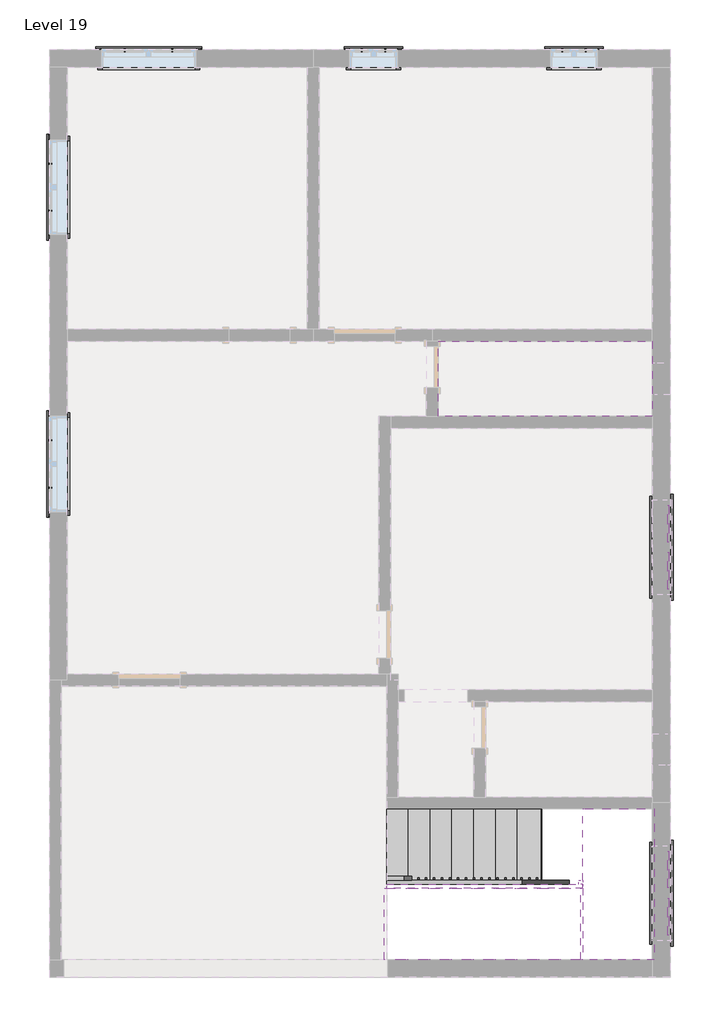
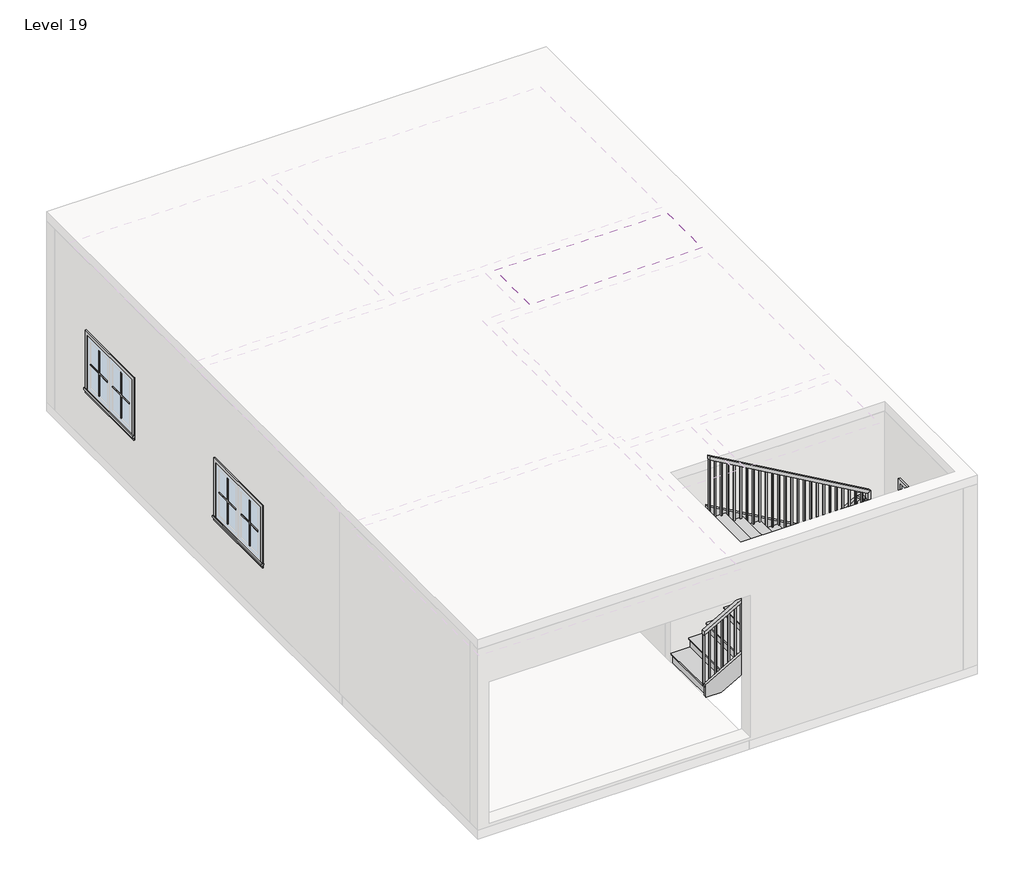
# One storey, part 2 of 2: 44 proxies, 3 members, 2 stair flights, 1 covering, 1 railing, 1 slab.
"""IFC4 building model written with IfcOpenShell, lengths in millimetres."""

from ifc_helpers import new_model, si_unit, frame, origin, place, context, project, spatial, polyline, outline, extrude, faceted_brep, transform, mapped, element, save
from components import muntin_pattern_2x2_muntin_pattern_2x2_2357e71d, muntin_pattern_2x2_muntin_pattern_2x2_302d8f29, muntin_pattern_2x2_muntin_pattern_2x2_53152e2c, muntin_pattern_2x2_muntin_pattern_2x2_e8f3e573, trim_window_exterior_flat_with_sill_c4e67c73, trim_window_exterior_flat_with_sill_a665a915, trim_window_interior_flat_picture_frame_cf1733af, trim_window_interior_flat_picture_frame_d485c387, non_monolithic_landing_13b6ecfc, stair_flight_45c7a08f, stair_flight_466e09e8

model = new_model("IFC4")

# Units and contexts
model_context = context("Model", 3, world=origin())
ifc_project = project(units=[si_unit("LENGTHUNIT", "METRE", prefix="MILLI")], contexts=[model_context])

# Site, building, storey
site = spatial("IfcSite", under=ifc_project)
building = spatial("IfcBuilding", under=site)
storey = spatial("IfcBuildingStorey", under=building, Name="Level 19", Elevation=12801.6)

# Proxies
placement = place(None, origin())
muntin_pattern_2x2_muntin_pattern_2x2_shape = muntin_pattern_2x2_muntin_pattern_2x2_2357e71d(model_context)
element("IfcBuildingElementProxy", 1, Name="Muntin Pattern_2x2 : Muntin Pattern_2x2", ObjectType="Muntin Pattern_2x2 : Muntin Pattern_2x2", at=placement, inside=storey, context=model_context, shape_type="MappedRepresentation", body=[
    mapped(muntin_pattern_2x2_muntin_pattern_2x2_shape, transform((-4942.3279463, 5897.3080275, 13785.85), x_axis=(1.0, 0.0, 0.0), y_axis=(0.0, 1.0, 0.0), z_axis=(0.0, 0.0, 1.0))),
])
element("IfcBuildingElementProxy", 2, Name="Muntin Pattern_2x2 : Muntin Pattern_2x2", ObjectType="Muntin Pattern_2x2 : Muntin Pattern_2x2", at=placement, inside=storey, context=model_context, shape_type="MappedRepresentation", body=[
    mapped(muntin_pattern_2x2_muntin_pattern_2x2_shape, transform((-5899.5904463, 3838.3205275, 13785.85), x_axis=(0.0, 1.0, 0.0), y_axis=(-1.0, 0.0, 0.0), z_axis=(0.0, 0.0, 1.0))),
])
element("IfcBuildingElementProxy", 3, Name="Muntin Pattern_2x2 : Muntin Pattern_2x2", ObjectType="Muntin Pattern_2x2 : Muntin Pattern_2x2", at=placement, inside=storey, context=model_context, shape_type="MappedRepresentation", body=[
    mapped(muntin_pattern_2x2_muntin_pattern_2x2_shape, transform((-5899.5904463, 293.4330275, 13785.85), x_axis=(0.0, 1.0, 0.0), y_axis=(-1.0, 0.0, 0.0), z_axis=(0.0, 0.0, 1.0))),
])
element("IfcBuildingElementProxy", 4, Name="Muntin Pattern_2x2 : Muntin Pattern_2x2", ObjectType="Muntin Pattern_2x2 : Muntin Pattern_2x2", at=placement, inside=storey, context=model_context, shape_type="MappedRepresentation", body=[
    mapped(muntin_pattern_2x2_muntin_pattern_2x2_shape, transform((2031.5595537, -166.9419725, 14090.65), x_axis=(0.0, -1.0, 0.0), y_axis=(1.0, 0.0, 0.0), z_axis=(0.0, 0.0, 1.0))),
])
element("IfcBuildingElementProxy", 5, Name="Muntin Pattern_2x2 : Muntin Pattern_2x2", ObjectType="Muntin Pattern_2x2 : Muntin Pattern_2x2", at=placement, inside=storey, context=model_context, shape_type="MappedRepresentation", body=[
    mapped(muntin_pattern_2x2_muntin_pattern_2x2_shape, transform((2031.5595537, -4599.2419725, 14090.65), x_axis=(0.0, -1.0, 0.0), y_axis=(1.0, 0.0, 0.0), z_axis=(0.0, 0.0, 1.0))),
])
element("IfcBuildingElementProxy", 6, Name="Muntin Pattern_2x2 : Muntin Pattern_2x2", ObjectType="Muntin Pattern_2x2 : Muntin Pattern_2x2", at=placement, inside=storey, context=model_context, shape_type="MappedRepresentation", body=[
    mapped(muntin_pattern_2x2_muntin_pattern_2x2_shape, transform((-4942.3279463, 5897.3080275, 13785.85), x_axis=(1.0, 0.0, 0.0), y_axis=(0.0, 1.0, 0.0), z_axis=(0.0, 0.0, 1.0))),
])
element("IfcBuildingElementProxy", 7, Name="Muntin Pattern_2x2 : Muntin Pattern_2x2", ObjectType="Muntin Pattern_2x2 : Muntin Pattern_2x2", at=placement, inside=storey, context=model_context, shape_type="MappedRepresentation", body=[
    mapped(muntin_pattern_2x2_muntin_pattern_2x2_shape, transform((2031.5595537, -4599.2419725, 14090.65), x_axis=(0.0, -1.0, 0.0), y_axis=(1.0, 0.0, 0.0), z_axis=(0.0, 0.0, 1.0))),
])
muntin_pattern_2x2_muntin_pattern_2x2_2_shape = muntin_pattern_2x2_muntin_pattern_2x2_302d8f29(model_context)
element("IfcBuildingElementProxy", 8, Name="Muntin Pattern_2x2 : Muntin Pattern_2x2", ObjectType="Muntin Pattern_2x2 : Muntin Pattern_2x2", at=placement, inside=storey, context=model_context, shape_type="MappedRepresentation", body=[
    mapped(muntin_pattern_2x2_muntin_pattern_2x2_2_shape, transform((-4335.9029463, 5897.3080275, 13785.85), x_axis=(-1.0, 0.0, 0.0), y_axis=(0.0, -1.0, 0.0), z_axis=(0.0, 0.0, 1.0))),
])
element("IfcBuildingElementProxy", 9, Name="Muntin Pattern_2x2 : Muntin Pattern_2x2", ObjectType="Muntin Pattern_2x2 : Muntin Pattern_2x2", at=placement, inside=storey, context=model_context, shape_type="MappedRepresentation", body=[
    mapped(muntin_pattern_2x2_muntin_pattern_2x2_2_shape, transform((-5899.5904463, 4444.7455275, 13785.85), x_axis=(0.0, -1.0, 0.0), y_axis=(1.0, 0.0, 0.0), z_axis=(0.0, 0.0, 1.0))),
])
element("IfcBuildingElementProxy", 10, Name="Muntin Pattern_2x2 : Muntin Pattern_2x2", ObjectType="Muntin Pattern_2x2 : Muntin Pattern_2x2", at=placement, inside=storey, context=model_context, shape_type="MappedRepresentation", body=[
    mapped(muntin_pattern_2x2_muntin_pattern_2x2_2_shape, transform((-5899.5904463, 899.8580275, 13785.85), x_axis=(0.0, -1.0, 0.0), y_axis=(1.0, 0.0, 0.0), z_axis=(0.0, 0.0, 1.0))),
])
element("IfcBuildingElementProxy", 11, Name="Muntin Pattern_2x2 : Muntin Pattern_2x2", ObjectType="Muntin Pattern_2x2 : Muntin Pattern_2x2", at=placement, inside=storey, context=model_context, shape_type="MappedRepresentation", body=[
    mapped(muntin_pattern_2x2_muntin_pattern_2x2_2_shape, transform((2031.5595537, -773.3669725, 14090.65), x_axis=(0.0, 1.0, 0.0), y_axis=(-1.0, 0.0, 0.0), z_axis=(0.0, 0.0, 1.0))),
])
element("IfcBuildingElementProxy", 12, Name="Muntin Pattern_2x2 : Muntin Pattern_2x2", ObjectType="Muntin Pattern_2x2 : Muntin Pattern_2x2", at=placement, inside=storey, context=model_context, shape_type="MappedRepresentation", body=[
    mapped(muntin_pattern_2x2_muntin_pattern_2x2_2_shape, transform((2031.5595537, -5205.6669725, 14090.65), x_axis=(0.0, 1.0, 0.0), y_axis=(-1.0, 0.0, 0.0), z_axis=(0.0, 0.0, 1.0))),
])
element("IfcBuildingElementProxy", 13, Name="Muntin Pattern_2x2 : Muntin Pattern_2x2", ObjectType="Muntin Pattern_2x2 : Muntin Pattern_2x2", at=placement, inside=storey, context=model_context, shape_type="MappedRepresentation", body=[
    mapped(muntin_pattern_2x2_muntin_pattern_2x2_2_shape, transform((-4335.9029463, 5897.3080275, 13785.85), x_axis=(-1.0, 0.0, 0.0), y_axis=(0.0, -1.0, 0.0), z_axis=(0.0, 0.0, 1.0))),
])
element("IfcBuildingElementProxy", 14, Name="Muntin Pattern_2x2 : Muntin Pattern_2x2", ObjectType="Muntin Pattern_2x2 : Muntin Pattern_2x2", at=placement, inside=storey, context=model_context, shape_type="MappedRepresentation", body=[
    mapped(muntin_pattern_2x2_muntin_pattern_2x2_2_shape, transform((2031.5595537, -5205.6669725, 14090.65), x_axis=(0.0, 1.0, 0.0), y_axis=(-1.0, 0.0, 0.0), z_axis=(0.0, 0.0, 1.0))),
])
muntin_pattern_2x2_muntin_pattern_2x2_3_shape = muntin_pattern_2x2_muntin_pattern_2x2_53152e2c(model_context)
element("IfcBuildingElementProxy", 15, Name="Muntin Pattern_2x2 : Muntin Pattern_2x2", ObjectType="Muntin Pattern_2x2 : Muntin Pattern_2x2", at=placement, inside=storey, context=model_context, shape_type="MappedRepresentation", body=[
    mapped(muntin_pattern_2x2_muntin_pattern_2x2_3_shape, transform((-1907.0279463, 5897.3080275, 13785.85), x_axis=(1.0, 0.0, 0.0), y_axis=(0.0, 1.0, 0.0), z_axis=(0.0, 0.0, 1.0))),
])
element("IfcBuildingElementProxy", 16, Name="Muntin Pattern_2x2 : Muntin Pattern_2x2", ObjectType="Muntin Pattern_2x2 : Muntin Pattern_2x2", at=placement, inside=storey, context=model_context, shape_type="MappedRepresentation", body=[
    mapped(muntin_pattern_2x2_muntin_pattern_2x2_3_shape, transform((658.3720537, 5897.3080275, 13785.85), x_axis=(1.0, 0.0, 0.0), y_axis=(0.0, 1.0, 0.0), z_axis=(0.0, 0.0, 1.0))),
])
element("IfcBuildingElementProxy", 17, Name="Muntin Pattern_2x2 : Muntin Pattern_2x2", ObjectType="Muntin Pattern_2x2 : Muntin Pattern_2x2", at=placement, inside=storey, context=model_context, shape_type="MappedRepresentation", body=[
    mapped(muntin_pattern_2x2_muntin_pattern_2x2_3_shape, transform((-1907.0279463, 5897.3080275, 13785.85), x_axis=(1.0, 0.0, 0.0), y_axis=(0.0, 1.0, 0.0), z_axis=(0.0, 0.0, 1.0))),
])
element("IfcBuildingElementProxy", 18, Name="Muntin Pattern_2x2 : Muntin Pattern_2x2", ObjectType="Muntin Pattern_2x2 : Muntin Pattern_2x2", at=placement, inside=storey, context=model_context, shape_type="MappedRepresentation", body=[
    mapped(muntin_pattern_2x2_muntin_pattern_2x2_3_shape, transform((658.3720537, 5897.3080275, 13785.85), x_axis=(1.0, 0.0, 0.0), y_axis=(0.0, 1.0, 0.0), z_axis=(0.0, 0.0, 1.0))),
])
muntin_pattern_2x2_muntin_pattern_2x2_4_shape = muntin_pattern_2x2_muntin_pattern_2x2_e8f3e573(model_context)
element("IfcBuildingElementProxy", 19, Name="Muntin Pattern_2x2 : Muntin Pattern_2x2", ObjectType="Muntin Pattern_2x2 : Muntin Pattern_2x2", at=placement, inside=storey, context=model_context, shape_type="MappedRepresentation", body=[
    mapped(muntin_pattern_2x2_muntin_pattern_2x2_4_shape, transform((-1605.4029463, 5897.3080275, 13785.85), x_axis=(-1.0, 0.0, 0.0), y_axis=(0.0, -1.0, 0.0), z_axis=(0.0, 0.0, 1.0))),
])
element("IfcBuildingElementProxy", 20, Name="Muntin Pattern_2x2 : Muntin Pattern_2x2", ObjectType="Muntin Pattern_2x2 : Muntin Pattern_2x2", at=placement, inside=storey, context=model_context, shape_type="MappedRepresentation", body=[
    mapped(muntin_pattern_2x2_muntin_pattern_2x2_4_shape, transform((959.9970537, 5897.3080275, 13785.85), x_axis=(-1.0, 0.0, 0.0), y_axis=(0.0, -1.0, 0.0), z_axis=(0.0, 0.0, 1.0))),
])
element("IfcBuildingElementProxy", 21, Name="Muntin Pattern_2x2 : Muntin Pattern_2x2", ObjectType="Muntin Pattern_2x2 : Muntin Pattern_2x2", at=placement, inside=storey, context=model_context, shape_type="MappedRepresentation", body=[
    mapped(muntin_pattern_2x2_muntin_pattern_2x2_4_shape, transform((-1605.4029463, 5897.3080275, 13785.85), x_axis=(-1.0, 0.0, 0.0), y_axis=(0.0, -1.0, 0.0), z_axis=(0.0, 0.0, 1.0))),
])
element("IfcBuildingElementProxy", 22, Name="Muntin Pattern_2x2 : Muntin Pattern_2x2", ObjectType="Muntin Pattern_2x2 : Muntin Pattern_2x2", at=placement, inside=storey, context=model_context, shape_type="MappedRepresentation", body=[
    mapped(muntin_pattern_2x2_muntin_pattern_2x2_4_shape, transform((959.9970537, 5897.3080275, 13785.85), x_axis=(-1.0, 0.0, 0.0), y_axis=(0.0, -1.0, 0.0), z_axis=(0.0, 0.0, 1.0))),
])
trim_window_exterior_flat_with_sill_shape = trim_window_exterior_flat_with_sill_c4e67c73(model_context)
element("IfcBuildingElementProxy", 23, Name="Trim-Window-Exterior-Flat : with Sill", ObjectType="Trim-Window-Exterior-Flat : with Sill", at=placement, inside=storey, context=model_context, shape_type="MappedRepresentation", body=[
    mapped(trim_window_exterior_flat_with_sill_shape, transform((-4639.1154463, 5906.8330275, 14630.4), x_axis=(-1.0, 0.0, 0.0), y_axis=(0.0, 0.0, 1.0), z_axis=(0.0, 1.0, 0.0))),
])
element("IfcBuildingElementProxy", 24, Name="Trim-Window-Exterior-Flat : with Sill", ObjectType="Trim-Window-Exterior-Flat : with Sill", at=placement, inside=storey, context=model_context, shape_type="MappedRepresentation", body=[
    mapped(trim_window_exterior_flat_with_sill_shape, transform((-5909.1154463, 4141.5330275, 14630.4), x_axis=(0.0, -1.0, 0.0), y_axis=(0.0, 0.0, 1.0), z_axis=(-1.0, 0.0, 0.0))),
])
element("IfcBuildingElementProxy", 25, Name="Trim-Window-Exterior-Flat : with Sill", ObjectType="Trim-Window-Exterior-Flat : with Sill", at=placement, inside=storey, context=model_context, shape_type="MappedRepresentation", body=[
    mapped(trim_window_exterior_flat_with_sill_shape, transform((-5909.1154463, 596.6455275, 14630.4), x_axis=(0.0, -1.0, 0.0), y_axis=(0.0, 0.0, 1.0), z_axis=(-1.0, 0.0, 0.0))),
])
element("IfcBuildingElementProxy", 26, Name="Trim-Window-Exterior-Flat : with Sill", ObjectType="Trim-Window-Exterior-Flat : with Sill", at=placement, inside=storey, context=model_context, shape_type="MappedRepresentation", body=[
    mapped(trim_window_exterior_flat_with_sill_shape, transform((2041.0845537, -470.1544725, 14935.2), x_axis=(0.0, 1.0, 0.0), y_axis=(0.0, 0.0, 1.0), z_axis=(1.0, 0.0, 0.0))),
])
element("IfcBuildingElementProxy", 27, Name="Trim-Window-Exterior-Flat : with Sill", ObjectType="Trim-Window-Exterior-Flat : with Sill", at=placement, inside=storey, context=model_context, shape_type="MappedRepresentation", body=[
    mapped(trim_window_exterior_flat_with_sill_shape, transform((2041.0845537, -4902.4544725, 14935.2), x_axis=(0.0, 1.0, 0.0), y_axis=(0.0, 0.0, 1.0), z_axis=(1.0, 0.0, 0.0))),
])
element("IfcBuildingElementProxy", 28, Name="Trim-Window-Exterior-Flat : with Sill", ObjectType="Trim-Window-Exterior-Flat : with Sill", at=placement, inside=storey, context=model_context, shape_type="MappedRepresentation", body=[
    mapped(trim_window_exterior_flat_with_sill_shape, transform((-4639.1154463, 5906.8330275, 14630.4), x_axis=(-1.0, 0.0, 0.0), y_axis=(0.0, 0.0, 1.0), z_axis=(0.0, 1.0, 0.0))),
])
element("IfcBuildingElementProxy", 29, Name="Trim-Window-Exterior-Flat : with Sill", ObjectType="Trim-Window-Exterior-Flat : with Sill", at=placement, inside=storey, context=model_context, shape_type="MappedRepresentation", body=[
    mapped(trim_window_exterior_flat_with_sill_shape, transform((2041.0845537, -4902.4544725, 14935.2), x_axis=(0.0, 1.0, 0.0), y_axis=(0.0, 0.0, 1.0), z_axis=(1.0, 0.0, 0.0))),
])
trim_window_exterior_flat_with_sill_2_shape = trim_window_exterior_flat_with_sill_a665a915(model_context)
element("IfcBuildingElementProxy", 30, Name="Trim-Window-Exterior-Flat : with Sill", ObjectType="Trim-Window-Exterior-Flat : with Sill", at=placement, inside=storey, context=model_context, shape_type="MappedRepresentation", body=[
    mapped(trim_window_exterior_flat_with_sill_2_shape, transform((-1756.2154463, 5906.8330275, 14630.4), x_axis=(-1.0, 0.0, 0.0), y_axis=(0.0, 0.0, 1.0), z_axis=(0.0, 1.0, 0.0))),
])
element("IfcBuildingElementProxy", 31, Name="Trim-Window-Exterior-Flat : with Sill", ObjectType="Trim-Window-Exterior-Flat : with Sill", at=placement, inside=storey, context=model_context, shape_type="MappedRepresentation", body=[
    mapped(trim_window_exterior_flat_with_sill_2_shape, transform((809.1845537, 5906.8330275, 14630.4), x_axis=(-1.0, 0.0, 0.0), y_axis=(0.0, 0.0, 1.0), z_axis=(0.0, 1.0, 0.0))),
])
element("IfcBuildingElementProxy", 32, Name="Trim-Window-Exterior-Flat : with Sill", ObjectType="Trim-Window-Exterior-Flat : with Sill", at=placement, inside=storey, context=model_context, shape_type="MappedRepresentation", body=[
    mapped(trim_window_exterior_flat_with_sill_2_shape, transform((-1756.2154463, 5906.8330275, 14630.4), x_axis=(-1.0, 0.0, 0.0), y_axis=(0.0, 0.0, 1.0), z_axis=(0.0, 1.0, 0.0))),
])
element("IfcBuildingElementProxy", 33, Name="Trim-Window-Exterior-Flat : with Sill", ObjectType="Trim-Window-Exterior-Flat : with Sill", at=placement, inside=storey, context=model_context, shape_type="MappedRepresentation", body=[
    mapped(trim_window_exterior_flat_with_sill_2_shape, transform((809.1845537, 5906.8330275, 14630.4), x_axis=(-1.0, 0.0, 0.0), y_axis=(0.0, 0.0, 1.0), z_axis=(0.0, 1.0, 0.0))),
])
trim_window_interior_flat_picture_frame_shape = trim_window_interior_flat_picture_frame_cf1733af(model_context)
element("IfcBuildingElementProxy", 34, Name="Trim-Window-Interior-Flat : Picture Frame", ObjectType="Trim-Window-Interior-Flat : Picture Frame", at=placement, inside=storey, context=model_context, shape_type="MappedRepresentation", body=[
    mapped(trim_window_interior_flat_picture_frame_shape, transform((-4639.1154463, 5678.2330275, 14630.4), x_axis=(1.0, 0.0, 0.0), y_axis=(0.0, 0.0, 1.0), z_axis=(0.0, -1.0, 0.0))),
])
element("IfcBuildingElementProxy", 35, Name="Trim-Window-Interior-Flat : Picture Frame", ObjectType="Trim-Window-Interior-Flat : Picture Frame", at=placement, inside=storey, context=model_context, shape_type="MappedRepresentation", body=[
    mapped(trim_window_interior_flat_picture_frame_shape, transform((-5680.5154463, 4141.5330275, 14630.4), x_axis=(0.0, 1.0, 0.0), y_axis=(0.0, 0.0, 1.0), z_axis=(1.0, 0.0, 0.0))),
])
element("IfcBuildingElementProxy", 36, Name="Trim-Window-Interior-Flat : Picture Frame", ObjectType="Trim-Window-Interior-Flat : Picture Frame", at=placement, inside=storey, context=model_context, shape_type="MappedRepresentation", body=[
    mapped(trim_window_interior_flat_picture_frame_shape, transform((-5680.5154463, 596.6455275, 14630.4), x_axis=(0.0, 1.0, 0.0), y_axis=(0.0, 0.0, 1.0), z_axis=(1.0, 0.0, 0.0))),
])
element("IfcBuildingElementProxy", 37, Name="Trim-Window-Interior-Flat : Picture Frame", ObjectType="Trim-Window-Interior-Flat : Picture Frame", at=placement, inside=storey, context=model_context, shape_type="MappedRepresentation", body=[
    mapped(trim_window_interior_flat_picture_frame_shape, transform((1812.4845537, -470.1544725, 14935.2), x_axis=(0.0, -1.0, 0.0), y_axis=(0.0, 0.0, 1.0), z_axis=(-1.0, 0.0, 0.0))),
])
element("IfcBuildingElementProxy", 38, Name="Trim-Window-Interior-Flat : Picture Frame", ObjectType="Trim-Window-Interior-Flat : Picture Frame", at=placement, inside=storey, context=model_context, shape_type="MappedRepresentation", body=[
    mapped(trim_window_interior_flat_picture_frame_shape, transform((1812.4845537, -4902.4544725, 14935.2), x_axis=(0.0, -1.0, 0.0), y_axis=(0.0, 0.0, 1.0), z_axis=(-1.0, 0.0, 0.0))),
])
element("IfcBuildingElementProxy", 39, Name="Trim-Window-Interior-Flat : Picture Frame", ObjectType="Trim-Window-Interior-Flat : Picture Frame", at=placement, inside=storey, context=model_context, shape_type="MappedRepresentation", body=[
    mapped(trim_window_interior_flat_picture_frame_shape, transform((-4639.1154463, 5678.2330275, 14630.4), x_axis=(1.0, 0.0, 0.0), y_axis=(0.0, 0.0, 1.0), z_axis=(0.0, -1.0, 0.0))),
])
element("IfcBuildingElementProxy", 40, Name="Trim-Window-Interior-Flat : Picture Frame", ObjectType="Trim-Window-Interior-Flat : Picture Frame", at=placement, inside=storey, context=model_context, shape_type="MappedRepresentation", body=[
    mapped(trim_window_interior_flat_picture_frame_shape, transform((1812.4845537, -4902.4544725, 14935.2), x_axis=(0.0, -1.0, 0.0), y_axis=(0.0, 0.0, 1.0), z_axis=(-1.0, 0.0, 0.0))),
])
trim_window_interior_flat_picture_frame_2_shape = trim_window_interior_flat_picture_frame_d485c387(model_context)
element("IfcBuildingElementProxy", 41, Name="Trim-Window-Interior-Flat : Picture Frame", ObjectType="Trim-Window-Interior-Flat : Picture Frame", at=placement, inside=storey, context=model_context, shape_type="MappedRepresentation", body=[
    mapped(trim_window_interior_flat_picture_frame_2_shape, transform((-1756.2154463, 5678.2330275, 14630.4), x_axis=(1.0, 0.0, 0.0), y_axis=(0.0, 0.0, 1.0), z_axis=(0.0, -1.0, 0.0))),
])
element("IfcBuildingElementProxy", 42, Name="Trim-Window-Interior-Flat : Picture Frame", ObjectType="Trim-Window-Interior-Flat : Picture Frame", at=placement, inside=storey, context=model_context, shape_type="MappedRepresentation", body=[
    mapped(trim_window_interior_flat_picture_frame_2_shape, transform((809.1845537, 5678.2330275, 14630.4), x_axis=(1.0, 0.0, 0.0), y_axis=(0.0, 0.0, 1.0), z_axis=(0.0, -1.0, 0.0))),
])
element("IfcBuildingElementProxy", 43, Name="Trim-Window-Interior-Flat : Picture Frame", ObjectType="Trim-Window-Interior-Flat : Picture Frame", at=placement, inside=storey, context=model_context, shape_type="MappedRepresentation", body=[
    mapped(trim_window_interior_flat_picture_frame_2_shape, transform((-1756.2154463, 5678.2330275, 14630.4), x_axis=(1.0, 0.0, 0.0), y_axis=(0.0, 0.0, 1.0), z_axis=(0.0, -1.0, 0.0))),
])
element("IfcBuildingElementProxy", 44, Name="Trim-Window-Interior-Flat : Picture Frame", ObjectType="Trim-Window-Interior-Flat : Picture Frame", at=placement, inside=storey, context=model_context, shape_type="MappedRepresentation", body=[
    mapped(trim_window_interior_flat_picture_frame_2_shape, transform((809.1845537, 5678.2330275, 14630.4), x_axis=(1.0, 0.0, 0.0), y_axis=(0.0, 0.0, 1.0), z_axis=(0.0, -1.0, 0.0))),
])

# Covering
element("IfcCovering", 45, ObjectType="2' x 4' ACT System", at=placement, inside=storey, context=model_context, shape_type="SweptSolid", body=[
    extrude(outline(polyline([(-930.7154463, 2171.4455275), (1812.4845537, 2171.4455275), (1812.4845537, 1206.2455275), (-930.7154463, 1206.2455275), (-930.7154463, 2171.4455275)])), frame((0.0, 0.0, 15544.8), z_axis=(0.0, 0.0, 1.0), x_axis=(1.0, 0.0, 0.0)), (0.0, 0.0, 1.0), 57.15),
])

# Members
element("IfcMember", 46, ObjectType="Stringer - 2\" Width", at=placement, inside=storey, context=model_context, shape_type="SweptSolid", body=[
    extrude(outline(polyline([(13010.6890626, -1591.1154463), (12801.6, -1591.1154463), (12801.6, -1342.8974141), (14070.524218, 872.6845537), (14421.7745172, 872.6845537), (13010.6890626, -1591.1154463)])), frame((0.0, -4788.1544725, 0.0), z_axis=(0.0, 1.0, 0.0), x_axis=(0.0, 0.0, 1.0)), (0.0, 0.0, 1.0), 50.8),
])
element("IfcMember", 47, ObjectType="Stringer - 2\" Width", at=placement, inside=storey, context=model_context, shape_type="SweptSolid", body=[
    extrude(outline(polyline([(14259.6387634, 923.4845537), (14610.8890626, 923.4845537), (16051.0690626, -1591.1154463), (15699.8187634, -1591.1154463), (14259.6387634, 923.4845537)])), frame((0.0, -4838.9544725, 0.0), z_axis=(0.0, 1.0, 0.0), x_axis=(0.0, 0.0, 1.0)), (0.0, 0.0, 1.0), 50.8),
])
element("IfcMember", 48, ObjectType="Stringer - 2\" Width", at=placement, inside=storey, context=model_context, shape_type="SweptSolid", body=[
    extrude(outline(polyline([(872.6845537, -4737.3544725), (923.4845537, -4737.3544725), (923.4845537, -4788.1544725), (872.6845537, -4788.1544725), (872.6845537, -4737.3544725)])), frame((0.0, 0.0, 14173.2), z_axis=(0.0, 0.0, 1.0), x_axis=(1.0, 0.0, 0.0)), (0.0, 0.0, 1.0), 304.8),
])

# Railing
element("IfcRailing", 49, ObjectType="Handrail - Rectangular", at=placement, inside=storey, context=model_context, shape_type="SolidModel", body=[
    faceted_brep([(-1591.1154463, -4686.5544725, 13876.02), (-1591.1154463, -4686.5544725, 13817.4782835), (-1591.1154463, -4737.3544725, 13817.4782835), (-1591.1154463, -4737.3544725, 13876.02), (847.2845537, -4686.5544725, 15272.5581818), (898.0845537, -4686.5544725, 15243.1110107), (898.0845537, -4737.3544725, 15243.1110107), (847.2845537, -4737.3544725, 15272.5581818), (847.2845537, -4686.5544725, 15316.2), (898.0845537, -4686.5544725, 15265.4), (898.0845537, -4737.3544725, 15265.4), (847.2845537, -4737.3544725, 15316.2), (974.2845537, -4686.5544725, 15316.2), (974.2845537, -4686.5544725, 15265.4), (923.4845537, -4737.3544725, 15265.4), (923.4845537, -4737.3544725, 15316.2), (974.2845537, -4813.5544725, 15316.2), (974.2845537, -4813.5544725, 15265.4), (923.4845537, -4813.5544725, 15265.4), (923.4845537, -4813.5544725, 15316.2), (974.2845537, -4838.9544725, 15316.2), (923.4845537, -4838.9544725, 15316.2), (923.4845537, -4889.7544725, 15265.4), (974.2845537, -4889.7544725, 15265.4)], [[[0, 1, 2, 3]], [[1, 0, 4, 5]], [[2, 1, 5, 6]], [[3, 2, 6, 7]], [[0, 3, 7, 4]], [[5, 4, 8, 9]], [[6, 5, 9, 10]], [[7, 6, 10, 11]], [[4, 7, 11, 8]], [[9, 8, 12, 13]], [[10, 9, 13, 14]], [[11, 10, 14, 15]], [[8, 11, 15, 12]], [[13, 12, 16, 17]], [[14, 13, 17, 18]], [[15, 14, 18, 19]], [[12, 15, 19, 16]], [[20, 21, 22, 23]], [[17, 16, 20, 23]], [[18, 17, 23, 22]], [[19, 18, 22, 21]], [[16, 19, 21, 20]]]),
    faceted_brep([(974.2845537, -4838.9544725, 15316.2), (974.2845537, -4889.7544725, 15265.4), (923.4845537, -4889.7544725, 15265.4), (923.4845537, -4838.9544725, 15316.2), (974.2845537, -4838.9544725, 15447.1254545), (923.4845537, -4838.9544725, 15417.6782835), (923.4845537, -4889.7544725, 15417.6782835), (974.2845537, -4889.7544725, 15447.1254545)], [[[0, 1, 2, 3]], [[4, 5, 6, 7]], [[1, 0, 4, 7]], [[2, 1, 7, 6]], [[3, 2, 6, 5]], [[0, 3, 5, 4]]]),
    faceted_brep([(974.2845537, -4889.7544725, 15447.1254545), (923.4845537, -4889.7544725, 15417.6782835), (923.4845537, -4838.9544725, 15417.6782835), (974.2845537, -4838.9544725, 15447.1254545), (-1591.1154463, -4889.7544725, 16916.4), (-1591.1154463, -4838.9544725, 16916.4), (-1591.1154463, -4838.9544725, 16857.8582835), (-1591.1154463, -4889.7544725, 16857.8582835)], [[[0, 1, 2, 3]], [[4, 5, 6, 7]], [[1, 0, 4, 7]], [[2, 1, 7, 6]], [[3, 2, 6, 5]], [[0, 3, 5, 4]]]),
    extrude(outline(polyline([(16794.2139653, -1479.9904463), (16805.1244198, -1499.0404463), (15841.98, -1499.0404463), (15841.98, -1479.9904463), (16794.2139653, -1479.9904463)])), frame((0.0, -4873.8794725, 0.0), z_axis=(0.0, 1.0, 0.0), x_axis=(0.0, 0.0, 1.0)), (0.0, 0.0, 1.0), 19.05),
    extrude(outline(polyline([(16736.0248744, -1378.3904463), (16746.9353289, -1397.4404463), (15841.98, -1397.4404463), (15841.98, -1378.3904463), (16736.0248744, -1378.3904463)])), frame((0.0, -4873.8794725, 0.0), z_axis=(0.0, 1.0, 0.0), x_axis=(0.0, 0.0, 1.0)), (0.0, 0.0, 1.0), 19.05),
    extrude(outline(polyline([(16677.8357835, -1276.7904463), (16688.746238, -1295.8404463), (15681.96, -1295.8404463), (15681.96, -1276.7904463), (16677.8357835, -1276.7904463)])), frame((0.0, -4873.8794725, 0.0), z_axis=(0.0, 1.0, 0.0), x_axis=(0.0, 0.0, 1.0)), (0.0, 0.0, 1.0), 19.05),
    extrude(outline(polyline([(16619.6466926, -1175.1904463), (16630.5571471, -1194.2404463), (15681.96, -1194.2404463), (15681.96, -1175.1904463), (16619.6466926, -1175.1904463)])), frame((0.0, -4873.8794725, 0.0), z_axis=(0.0, 1.0, 0.0), x_axis=(0.0, 0.0, 1.0)), (0.0, 0.0, 1.0), 19.05),
    extrude(outline(polyline([(16561.4576016, -1073.5904463), (16572.3680562, -1092.6404463), (15681.96, -1092.6404463), (15681.96, -1073.5904463), (16561.4576016, -1073.5904463)])), frame((0.0, -4873.8794725, 0.0), z_axis=(0.0, 1.0, 0.0), x_axis=(0.0, 0.0, 1.0)), (0.0, 0.0, 1.0), 19.05),
    extrude(outline(polyline([(16503.2685107, -971.9904463), (16514.1789653, -991.0404463), (15521.94, -991.0404463), (15521.94, -971.9904463), (16503.2685107, -971.9904463)])), frame((0.0, -4873.8794725, 0.0), z_axis=(0.0, 1.0, 0.0), x_axis=(0.0, 0.0, 1.0)), (0.0, 0.0, 1.0), 19.05),
    extrude(outline(polyline([(16445.0794198, -870.3904463), (16455.9898744, -889.4404463), (15521.94, -889.4404463), (15521.94, -870.3904463), (16445.0794198, -870.3904463)])), frame((0.0, -4873.8794725, 0.0), z_axis=(0.0, 1.0, 0.0), x_axis=(0.0, 0.0, 1.0)), (0.0, 0.0, 1.0), 19.05),
    extrude(outline(polyline([(16386.8903289, -768.7904463), (16397.8007835, -787.8404463), (15521.94, -787.8404463), (15521.94, -768.7904463), (16386.8903289, -768.7904463)])), frame((0.0, -4873.8794725, 0.0), z_axis=(0.0, 1.0, 0.0), x_axis=(0.0, 0.0, 1.0)), (0.0, 0.0, 1.0), 19.05),
    extrude(outline(polyline([(16328.701238, -667.1904463), (16339.6116926, -686.2404463), (15361.92, -686.2404463), (15361.92, -667.1904463), (16328.701238, -667.1904463)])), frame((0.0, -4873.8794725, 0.0), z_axis=(0.0, 1.0, 0.0), x_axis=(0.0, 0.0, 1.0)), (0.0, 0.0, 1.0), 19.05),
    extrude(outline(polyline([(16270.5121471, -565.5904463), (16281.4226016, -584.6404463), (15361.92, -584.6404463), (15361.92, -565.5904463), (16270.5121471, -565.5904463)])), frame((0.0, -4873.8794725, 0.0), z_axis=(0.0, 1.0, 0.0), x_axis=(0.0, 0.0, 1.0)), (0.0, 0.0, 1.0), 19.05),
    extrude(outline(polyline([(16212.3230562, -463.9904463), (16223.2335107, -483.0404463), (15361.92, -483.0404463), (15361.92, -463.9904463), (16212.3230562, -463.9904463)])), frame((0.0, -4873.8794725, 0.0), z_axis=(0.0, 1.0, 0.0), x_axis=(0.0, 0.0, 1.0)), (0.0, 0.0, 1.0), 19.05),
    extrude(outline(polyline([(16154.1339653, -362.3904463), (16165.0444198, -381.4404463), (15201.9, -381.4404463), (15201.9, -362.3904463), (16154.1339653, -362.3904463)])), frame((0.0, -4873.8794725, 0.0), z_axis=(0.0, 1.0, 0.0), x_axis=(0.0, 0.0, 1.0)), (0.0, 0.0, 1.0), 19.05),
    extrude(outline(polyline([(16095.9448744, -260.7904463), (16106.8553289, -279.8404463), (15201.9, -279.8404463), (15201.9, -260.7904463), (16095.9448744, -260.7904463)])), frame((0.0, -4873.8794725, 0.0), z_axis=(0.0, 1.0, 0.0), x_axis=(0.0, 0.0, 1.0)), (0.0, 0.0, 1.0), 19.05),
    extrude(outline(polyline([(16037.7557835, -159.1904463), (16048.666238, -178.2404463), (15041.88, -178.2404463), (15041.88, -159.1904463), (16037.7557835, -159.1904463)])), frame((0.0, -4873.8794725, 0.0), z_axis=(0.0, 1.0, 0.0), x_axis=(0.0, 0.0, 1.0)), (0.0, 0.0, 1.0), 19.05),
    extrude(outline(polyline([(15979.5666926, -57.5904463), (15990.4771471, -76.6404463), (15041.88, -76.6404463), (15041.88, -57.5904463), (15979.5666926, -57.5904463)])), frame((0.0, -4873.8794725, 0.0), z_axis=(0.0, 1.0, 0.0), x_axis=(0.0, 0.0, 1.0)), (0.0, 0.0, 1.0), 19.05),
    extrude(outline(polyline([(15921.3776016, 44.0095537), (15932.2880562, 24.9595537), (15041.88, 24.9595537), (15041.88, 44.0095537), (15921.3776016, 44.0095537)])), frame((0.0, -4873.8794725, 0.0), z_axis=(0.0, 1.0, 0.0), x_axis=(0.0, 0.0, 1.0)), (0.0, 0.0, 1.0), 19.05),
    extrude(outline(polyline([(15863.1885107, 145.6095537), (15874.0989653, 126.5595537), (14881.86, 126.5595537), (14881.86, 145.6095537), (15863.1885107, 145.6095537)])), frame((0.0, -4873.8794725, 0.0), z_axis=(0.0, 1.0, 0.0), x_axis=(0.0, 0.0, 1.0)), (0.0, 0.0, 1.0), 19.05),
    extrude(outline(polyline([(15804.9994198, 247.2095537), (15815.9098744, 228.1595537), (14881.86, 228.1595537), (14881.86, 247.2095537), (15804.9994198, 247.2095537)])), frame((0.0, -4873.8794725, 0.0), z_axis=(0.0, 1.0, 0.0), x_axis=(0.0, 0.0, 1.0)), (0.0, 0.0, 1.0), 19.05),
    extrude(outline(polyline([(15746.8103289, 348.8095537), (15757.7207835, 329.7595537), (14881.86, 329.7595537), (14881.86, 348.8095537), (15746.8103289, 348.8095537)])), frame((0.0, -4873.8794725, 0.0), z_axis=(0.0, 1.0, 0.0), x_axis=(0.0, 0.0, 1.0)), (0.0, 0.0, 1.0), 19.05),
    extrude(outline(polyline([(15688.621238, 450.4095537), (15699.5316926, 431.3595537), (14721.84, 431.3595537), (14721.84, 450.4095537), (15688.621238, 450.4095537)])), frame((0.0, -4873.8794725, 0.0), z_axis=(0.0, 1.0, 0.0), x_axis=(0.0, 0.0, 1.0)), (0.0, 0.0, 1.0), 19.05),
    extrude(outline(polyline([(15630.4321471, 552.0095537), (15641.3426016, 532.9595537), (14721.84, 532.9595537), (14721.84, 552.0095537), (15630.4321471, 552.0095537)])), frame((0.0, -4873.8794725, 0.0), z_axis=(0.0, 1.0, 0.0), x_axis=(0.0, 0.0, 1.0)), (0.0, 0.0, 1.0), 19.05),
    extrude(outline(polyline([(15572.2430562, 653.6095537), (15583.1535107, 634.5595537), (14721.84, 634.5595537), (14721.84, 653.6095537), (15572.2430562, 653.6095537)])), frame((0.0, -4873.8794725, 0.0), z_axis=(0.0, 1.0, 0.0), x_axis=(0.0, 0.0, 1.0)), (0.0, 0.0, 1.0), 19.05),
    extrude(outline(polyline([(15514.0539653, 755.2095537), (15524.9644198, 736.1595537), (14561.82, 736.1595537), (14561.82, 755.2095537), (15514.0539653, 755.2095537)])), frame((0.0, -4873.8794725, 0.0), z_axis=(0.0, 1.0, 0.0), x_axis=(0.0, 0.0, 1.0)), (0.0, 0.0, 1.0), 19.05),
    extrude(outline(polyline([(15455.8648744, 856.8095537), (15466.7753289, 837.7595537), (14561.82, 837.7595537), (14561.82, 856.8095537), (15455.8648744, 856.8095537)])), frame((0.0, -4873.8794725, 0.0), z_axis=(0.0, 1.0, 0.0), x_axis=(0.0, 0.0, 1.0)), (0.0, 0.0, 1.0), 19.05),
    extrude(outline(polyline([(939.3595537, -4804.0294725), (958.4095537, -4804.0294725), (958.4095537, -4823.0794725), (939.3595537, -4823.0794725), (939.3595537, -4804.0294725)])), frame((0.0, 0.0, 14401.8), z_axis=(0.0, 0.0, 1.0), x_axis=(1.0, 0.0, 0.0)), (0.0, 0.0, 1.0), 863.6),
    extrude(outline(polyline([(15219.4716926, 856.8095537), (15208.561238, 837.7595537), (14241.78, 837.7595537), (14241.78, 856.8095537), (15219.4716926, 856.8095537)])), frame((0.0, -4721.4794725, 0.0), z_axis=(0.0, 1.0, 0.0), x_axis=(0.0, 0.0, 1.0)), (0.0, 0.0, 1.0), 19.05),
    extrude(outline(polyline([(15161.2826016, 755.2095537), (15150.3721471, 736.1595537), (14241.78, 736.1595537), (14241.78, 755.2095537), (15161.2826016, 755.2095537)])), frame((0.0, -4721.4794725, 0.0), z_axis=(0.0, 1.0, 0.0), x_axis=(0.0, 0.0, 1.0)), (0.0, 0.0, 1.0), 19.05),
    extrude(outline(polyline([(15103.0935107, 653.6095537), (15092.1830562, 634.5595537), (14241.78, 634.5595537), (14241.78, 653.6095537), (15103.0935107, 653.6095537)])), frame((0.0, -4721.4794725, 0.0), z_axis=(0.0, 1.0, 0.0), x_axis=(0.0, 0.0, 1.0)), (0.0, 0.0, 1.0), 19.05),
    extrude(outline(polyline([(15044.9044198, 552.0095537), (15033.9939653, 532.9595537), (14081.76, 532.9595537), (14081.76, 552.0095537), (15044.9044198, 552.0095537)])), frame((0.0, -4721.4794725, 0.0), z_axis=(0.0, 1.0, 0.0), x_axis=(0.0, 0.0, 1.0)), (0.0, 0.0, 1.0), 19.05),
    extrude(outline(polyline([(14986.7153289, 450.4095537), (14975.8048744, 431.3595537), (14081.76, 431.3595537), (14081.76, 450.4095537), (14986.7153289, 450.4095537)])), frame((0.0, -4721.4794725, 0.0), z_axis=(0.0, 1.0, 0.0), x_axis=(0.0, 0.0, 1.0)), (0.0, 0.0, 1.0), 19.05),
    extrude(outline(polyline([(14928.526238, 348.8095537), (14917.6157835, 329.7595537), (13921.74, 329.7595537), (13921.74, 348.8095537), (14928.526238, 348.8095537)])), frame((0.0, -4721.4794725, 0.0), z_axis=(0.0, 1.0, 0.0), x_axis=(0.0, 0.0, 1.0)), (0.0, 0.0, 1.0), 19.05),
    extrude(outline(polyline([(14870.3371471, 247.2095537), (14859.4266926, 228.1595537), (13921.74, 228.1595537), (13921.74, 247.2095537), (14870.3371471, 247.2095537)])), frame((0.0, -4721.4794725, 0.0), z_axis=(0.0, 1.0, 0.0), x_axis=(0.0, 0.0, 1.0)), (0.0, 0.0, 1.0), 19.05),
    extrude(outline(polyline([(14812.1480562, 145.6095537), (14801.2376016, 126.5595537), (13921.74, 126.5595537), (13921.74, 145.6095537), (14812.1480562, 145.6095537)])), frame((0.0, -4721.4794725, 0.0), z_axis=(0.0, 1.0, 0.0), x_axis=(0.0, 0.0, 1.0)), (0.0, 0.0, 1.0), 19.05),
    extrude(outline(polyline([(14753.9589653, 44.0095537), (14743.0485107, 24.9595537), (13761.72, 24.9595537), (13761.72, 44.0095537), (14753.9589653, 44.0095537)])), frame((0.0, -4721.4794725, 0.0), z_axis=(0.0, 1.0, 0.0), x_axis=(0.0, 0.0, 1.0)), (0.0, 0.0, 1.0), 19.05),
    extrude(outline(polyline([(14695.7698744, -57.5904463), (14684.8594198, -76.6404463), (13761.72, -76.6404463), (13761.72, -57.5904463), (14695.7698744, -57.5904463)])), frame((0.0, -4721.4794725, 0.0), z_axis=(0.0, 1.0, 0.0), x_axis=(0.0, 0.0, 1.0)), (0.0, 0.0, 1.0), 19.05),
    extrude(outline(polyline([(14637.5807835, -159.1904463), (14626.6703289, -178.2404463), (13761.72, -178.2404463), (13761.72, -159.1904463), (14637.5807835, -159.1904463)])), frame((0.0, -4721.4794725, 0.0), z_axis=(0.0, 1.0, 0.0), x_axis=(0.0, 0.0, 1.0)), (0.0, 0.0, 1.0), 19.05),
    extrude(outline(polyline([(14579.3916926, -260.7904463), (14568.481238, -279.8404463), (13601.7, -279.8404463), (13601.7, -260.7904463), (14579.3916926, -260.7904463)])), frame((0.0, -4721.4794725, 0.0), z_axis=(0.0, 1.0, 0.0), x_axis=(0.0, 0.0, 1.0)), (0.0, 0.0, 1.0), 19.05),
    extrude(outline(polyline([(14521.2026016, -362.3904463), (14510.2921471, -381.4404463), (13601.7, -381.4404463), (13601.7, -362.3904463), (14521.2026016, -362.3904463)])), frame((0.0, -4721.4794725, 0.0), z_axis=(0.0, 1.0, 0.0), x_axis=(0.0, 0.0, 1.0)), (0.0, 0.0, 1.0), 19.05),
    extrude(outline(polyline([(14463.0135107, -463.9904463), (14452.1030562, -483.0404463), (13601.7, -483.0404463), (13601.7, -463.9904463), (14463.0135107, -463.9904463)])), frame((0.0, -4721.4794725, 0.0), z_axis=(0.0, 1.0, 0.0), x_axis=(0.0, 0.0, 1.0)), (0.0, 0.0, 1.0), 19.05),
    extrude(outline(polyline([(14404.8244198, -565.5904463), (14393.9139653, -584.6404463), (13441.68, -584.6404463), (13441.68, -565.5904463), (14404.8244198, -565.5904463)])), frame((0.0, -4721.4794725, 0.0), z_axis=(0.0, 1.0, 0.0), x_axis=(0.0, 0.0, 1.0)), (0.0, 0.0, 1.0), 19.05),
    extrude(outline(polyline([(14346.6353289, -667.1904463), (14335.7248744, -686.2404463), (13441.68, -686.2404463), (13441.68, -667.1904463), (14346.6353289, -667.1904463)])), frame((0.0, -4721.4794725, 0.0), z_axis=(0.0, 1.0, 0.0), x_axis=(0.0, 0.0, 1.0)), (0.0, 0.0, 1.0), 19.05),
    extrude(outline(polyline([(14288.446238, -768.7904463), (14277.5357835, -787.8404463), (13281.66, -787.8404463), (13281.66, -768.7904463), (14288.446238, -768.7904463)])), frame((0.0, -4721.4794725, 0.0), z_axis=(0.0, 1.0, 0.0), x_axis=(0.0, 0.0, 1.0)), (0.0, 0.0, 1.0), 19.05),
    extrude(outline(polyline([(14230.2571471, -870.3904463), (14219.3466926, -889.4404463), (13281.66, -889.4404463), (13281.66, -870.3904463), (14230.2571471, -870.3904463)])), frame((0.0, -4721.4794725, 0.0), z_axis=(0.0, 1.0, 0.0), x_axis=(0.0, 0.0, 1.0)), (0.0, 0.0, 1.0), 19.05),
    extrude(outline(polyline([(14172.0680562, -971.9904463), (14161.1576016, -991.0404463), (13281.66, -991.0404463), (13281.66, -971.9904463), (14172.0680562, -971.9904463)])), frame((0.0, -4721.4794725, 0.0), z_axis=(0.0, 1.0, 0.0), x_axis=(0.0, 0.0, 1.0)), (0.0, 0.0, 1.0), 19.05),
    extrude(outline(polyline([(14113.8789653, -1073.5904463), (14102.9685107, -1092.6404463), (13121.64, -1092.6404463), (13121.64, -1073.5904463), (14113.8789653, -1073.5904463)])), frame((0.0, -4721.4794725, 0.0), z_axis=(0.0, 1.0, 0.0), x_axis=(0.0, 0.0, 1.0)), (0.0, 0.0, 1.0), 19.05),
    extrude(outline(polyline([(14055.6898744, -1175.1904463), (14044.7794198, -1194.2404463), (13121.64, -1194.2404463), (13121.64, -1175.1904463), (14055.6898744, -1175.1904463)])), frame((0.0, -4721.4794725, 0.0), z_axis=(0.0, 1.0, 0.0), x_axis=(0.0, 0.0, 1.0)), (0.0, 0.0, 1.0), 19.05),
    extrude(outline(polyline([(13997.5007835, -1276.7904463), (13986.5903289, -1295.8404463), (13121.64, -1295.8404463), (13121.64, -1276.7904463), (13997.5007835, -1276.7904463)])), frame((0.0, -4721.4794725, 0.0), z_axis=(0.0, 1.0, 0.0), x_axis=(0.0, 0.0, 1.0)), (0.0, 0.0, 1.0), 19.05),
    extrude(outline(polyline([(13939.3116926, -1378.3904463), (13928.401238, -1397.4404463), (12961.62, -1397.4404463), (12961.62, -1378.3904463), (13939.3116926, -1378.3904463)])), frame((0.0, -4721.4794725, 0.0), z_axis=(0.0, 1.0, 0.0), x_axis=(0.0, 0.0, 1.0)), (0.0, 0.0, 1.0), 19.05),
    extrude(outline(polyline([(13881.1226016, -1479.9904463), (13870.2121471, -1499.0404463), (12961.62, -1499.0404463), (12961.62, -1479.9904463), (13881.1226016, -1479.9904463)])), frame((0.0, -4721.4794725, 0.0), z_axis=(0.0, 1.0, 0.0), x_axis=(0.0, 0.0, 1.0)), (0.0, 0.0, 1.0), 19.05),
    extrude(outline(polyline([(939.3595537, -4854.8294725), (958.4095537, -4854.8294725), (958.4095537, -4873.8794725), (939.3595537, -4873.8794725), (939.3595537, -4854.8294725)])), frame((0.0, 0.0, 14401.8), z_axis=(0.0, 0.0, 1.0), x_axis=(1.0, 0.0, 0.0)), (0.0, 0.0, 1.0), 863.6),
    extrude(outline(polyline([(939.3595537, -4721.4794725), (939.3595537, -4702.4294725), (958.4095537, -4702.4294725), (958.4095537, -4721.4794725), (939.3595537, -4721.4794725)])), frame((0.0, 0.0, 14401.8), z_axis=(0.0, 0.0, 1.0), x_axis=(1.0, 0.0, 0.0)), (0.0, 0.0, 1.0), 863.6),
    extrude(outline(polyline([(16846.9478289, -1572.0654463), (16857.8582835, -1591.1154463), (15841.98, -1591.1154463), (15841.98, -1572.0654463), (16846.9478289, -1572.0654463)])), frame((0.0, -4873.8794725, 0.0), z_axis=(0.0, 1.0, 0.0), x_axis=(0.0, 0.0, 1.0)), (0.0, 0.0, 1.0), 19.05),
    extrude(outline(polyline([(13828.388738, -1572.0654463), (13817.4782835, -1591.1154463), (12961.62, -1591.1154463), (12961.62, -1572.0654463), (13828.388738, -1572.0654463)])), frame((0.0, -4721.4794725, 0.0), z_axis=(0.0, 1.0, 0.0), x_axis=(0.0, 0.0, 1.0)), (0.0, 0.0, 1.0), 19.05),
])

# Slab
non_monolithic_landing_shape = non_monolithic_landing_13b6ecfc(model_context)
element("IfcSlab", 50, ObjectType="Non-Monolithic Landing", at=placement, inside=storey, context=model_context, shape_type="MappedRepresentation", body=[
    mapped(non_monolithic_landing_shape, transform((0.0, 0.0, 0.0), x_axis=(1.0, 0.0, 0.0), y_axis=(0.0, 1.0, 0.0), z_axis=(0.0, 0.0, 1.0))),
])

# Stair flights
stair_flight_shape = stair_flight_45c7a08f(model_context)
element("IfcStairFlight", 51, ObjectType="2\" Tread 1\" Nosing 1/4\" Riser", at=placement, inside=storey, context=model_context, shape_type="MappedRepresentation", body=[
    mapped(stair_flight_shape, transform((0.0, 0.0, 0.0), x_axis=(1.0, 0.0, 0.0), y_axis=(0.0, 1.0, 0.0), z_axis=(0.0, 0.0, 1.0))),
])
stair_flight_2_shape = stair_flight_466e09e8(model_context)
element("IfcStairFlight", 52, ObjectType="2\" Tread 1\" Nosing 1/4\" Riser", at=placement, inside=storey, context=model_context, shape_type="MappedRepresentation", body=[
    mapped(stair_flight_2_shape, transform((0.0, 0.0, 0.0), x_axis=(1.0, 0.0, 0.0), y_axis=(0.0, 1.0, 0.0), z_axis=(0.0, 0.0, 1.0))),
])

save(model, "model.ifc")

# Revit data of these elements
# Type "Muntin Pattern_2x2 : Muntin Pattern_2x2"
#   Width [instance default] = 4' - 0"
#   Thickness = 0' - 0 1/2"
#   Height [instance default] = 4' - 0"
#   Distance = 0' - 0 3/4"
#   Interior Material [instance default] = none
#   Exterior Material [instance default] = none
#   Default Elevation = 0
# Type "Trim-Window-Exterior-Flat : with Sill"
#   Trim Width = 0' - 2 1/4"
#   Trim Thickness_Picture Frame = 0' - 1 1/4"
#   Trim Thickness_with Sill = 0' - 0 3/4"
#   Sill Thickness = 0' - 1 1/4"
#   Opening Width [instance default] = 2' - 0"
#   Opening Height [instance default] = 3' - 0"
#   Default Elevation = 4' - 0"
#   Sill = yes
#   Picture Frame = no
#   Trim Material [instance default] = none
# Type "Trim-Window-Interior-Flat : Picture Frame"
#   Trim Thickness_Picture Frame = 0' - 1 1/4"
#   Trim Width = 0' - 2 1/4"
#   Trim Thickness_with Sill = 0' - 0 3/4"
#   Sill Thickness = 0' - 1 1/4"
#   Opening Width [instance default] = 2' - 0"
#   Opening Height [instance default] = 3' - 0"
#   Default Elevation = 4' - 0"
#   Sill = no
#   Picture Frame = yes
#   Trim Material [instance default] = none
# Type "2' x 4' ACT System"
#   Assembly Code = "C3030210"
#   built-in parameter 1002203 = 1 (stored number, unit not read)
#   built-in parameter 1002202 = 1 (stored number, unit not read)
#   Layers, outside or top first: 0' - 1 5/8" "Default" (function 1); 0' - 0 5/8" "Acoustic Ceiling Tile 24 x 48" (function 5)
# Type "Handrail - Rectangular"
#   Assembly Code = "C2010400"
#   built-in parameter 1008612 = 0.0416667 (stored number, unit not read)
#   built-in parameter 1008611 = 0.0416667 (stored number, unit not read)
#   built-in parameter 1008609 = 0.333333 (stored number, unit not read)
#   built-in parameter 1008604 = 0.166667 (stored number, unit not read)
#   built-in parameter 1008603 = 0.166667 (stored number, unit not read)
#   Railing Height = 3' - 0"
#   built-in parameter 1008630 = 2
#   built-in parameter 1008610 = 2
#   built-in parameter 1008618 = Baluster - Square : 3/4"
# Elements 1, 2, 3, 4, 5, 6, 7, 8, 9, 10, 11, 12, 13, 14 (IfcBuildingElementProxy, "Muntin Pattern_2x2 : Muntin Pattern_2x2")
#   Width = 1' - 6 5/8"
#   Height = 2' - 6 1/2"
#   Interior Material = Wood - Stained
#   Exterior Material = Clad - White
#   Phase Created = New Construction
#   Materials on its faces: "Clad - White", "Wood - Stained"
# Elements 15, 16, 17, 18, 19, 20, 21, 22 (IfcBuildingElementProxy, "Muntin Pattern_2x2 : Muntin Pattern_2x2")
#   Width = 0' - 6 5/8"
#   Height = 2' - 6 1/2"
#   Interior Material = Wood - Stained
#   Exterior Material = Clad - White
#   Phase Created = New Construction
#   Materials on its faces: "Clad - White", "Wood - Stained"
# Elements 23, 24, 25, 26, 27, 28, 29 (IfcBuildingElementProxy, "Trim-Window-Exterior-Flat : with Sill")
#   Opening Width = 4' - 0"
#   Opening Height = 3' - 0"
#   Trim Material = Clad - White
#   Phase Created = New Construction
#   Materials on its faces: "Clad - White"
# Elements 30, 31, 32, 33 (IfcBuildingElementProxy, "Trim-Window-Exterior-Flat : with Sill")
#   Opening Width = 2' - 0"
#   Opening Height = 3' - 0"
#   Trim Material = Clad - White
#   Phase Created = New Construction
#   Materials on its faces: "Clad - White"
# Elements 34, 35, 36, 37, 38, 39, 40 (IfcBuildingElementProxy, "Trim-Window-Interior-Flat : Picture Frame")
#   Opening Width = 4' - 0"
#   Opening Height = 3' - 0"
#   Trim Material = Wood - Stained
#   Phase Created = New Construction
#   Materials on its faces: "Wood - Stained"
# Elements 41, 42, 43, 44 (IfcBuildingElementProxy, "Trim-Window-Interior-Flat : Picture Frame")
#   Opening Width = 2' - 0"
#   Opening Height = 3' - 0"
#   Trim Material = Wood - Stained
#   Phase Created = New Construction
#   Materials on its faces: "Wood - Stained"
# Element 45 (IfcCovering, "2' x 4' ACT System")
#   Height Offset From Level = 9' - 0"
#   Phase Created = New Construction
#   Materials on its faces: "Acoustic Ceiling Tile 24 x 48", "Default"
# Elements 46, 47, 48 (IfcMember, "Stringer - 2\" Width")
#   Phase Created = New Construction
# Element 49 (IfcRailing, "Handrail - Rectangular")
#   Phase Created = New Construction
# Element 50 (IfcSlab, "Non-Monolithic Landing")
#   Phase Created = New Construction
# Elements 51, 52 (IfcStairFlight, "2\" Tread 1\" Nosing 1/4\" Riser")
#   Phase Created = New Construction
# Materials
#   "Default": colour RGB 127 127 127, transparency 0, Cost = 0
#   "Acoustic Ceiling Tile 24 x 48": class "Generic", colour RGB 229 229 229, transparency 0, Description = "Acoustic Ceiling Tile 24 x 48", Cost = 0
#   "Clad - White": class "Wood", colour RGB 242 242 238, transparency 0, Cost = 0
#   "Wood - Stained": class "Wood", colour RGB 224 178 126, transparency 0, Cost = 0
